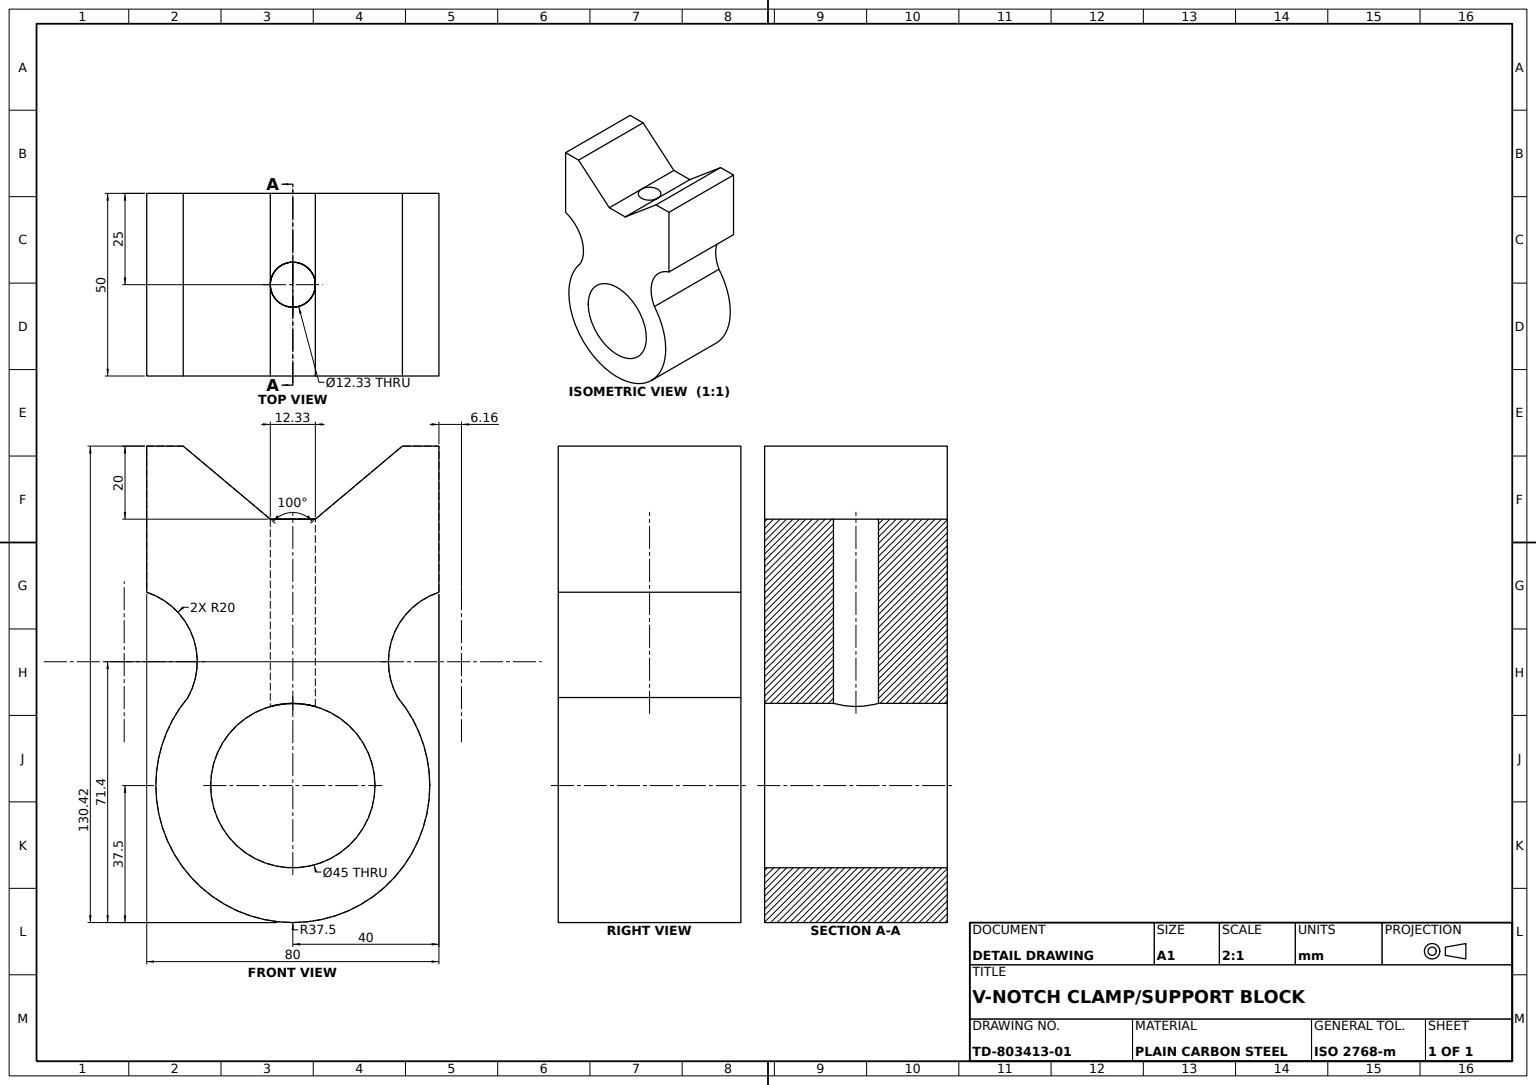
from build123d import *

# Parameters (mm, degrees)
V_BLOCK_PROFILE_SKETCH_R = 22.5
V_BLOCK_BODY_DEPTH       = 25
CROSS_HOLE_SKETCH_R      = 6.164856296
CROSS_HOLE_DEPTH         = 60


with BuildPart() as part:
    # V-Block Profile Sketch → V-Block Body (new, symmetric)
    with BuildSketch(Plane.XY):
        with BuildLine():
            Line((-40.000071852, 52.924513188), (-40.000071852, 92.924513188))
            Line((-40.000071852, 92.924513188), (-30.000071852, 92.924513188))
            Line((-30.000071852, 92.924513188), (-6.165, 72.924513188))
            Line((-6.165, 72.924513188), (6.164856296, 72.924513188))
            Line((6.164856296, 72.924513188), (29.999928148, 92.924513188))
            Line((29.999928148, 92.924513188), (39.999928148, 92.924513188))
            Line((39.999928148, 92.924513188), (39.999928148, 52.924513188))
            ThreePointArc((39.999928148, 52.924513188), (27.538857009, 41.183981608), (28.726666617, 24.104535363))
            ThreePointArc((28.726666617, 24.104535363), (0, -37.5), (-28.726666617, 24.104535363))
            ThreePointArc((-28.726666617, 24.104535363), (-27.538910641, 41.184022764), (-40.000071852, 52.924513188))
        make_face()
        Circle(V_BLOCK_PROFILE_SKETCH_R, mode=Mode.SUBTRACT)
    extrude(amount=V_BLOCK_BODY_DEPTH, both=True)

    # Cross Hole Sketch → Cross Hole (cut)
    with BuildSketch(Plane(origin=(0, 72.924513188, 0), x_dir=(1, 0, 0), z_dir=(0, 1, 0))):
        with Locations(Location((0, 0, 0), (0, 0, 270))):
            Circle(CROSS_HOLE_SKETCH_R)
    extrude(amount=-CROSS_HOLE_DEPTH, mode=Mode.SUBTRACT)


solid = part.part
